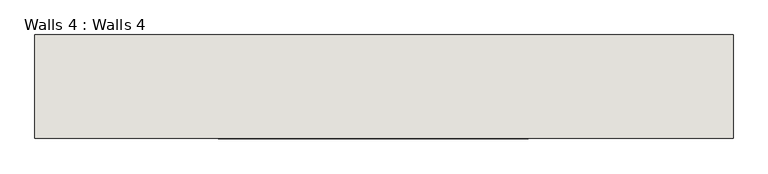
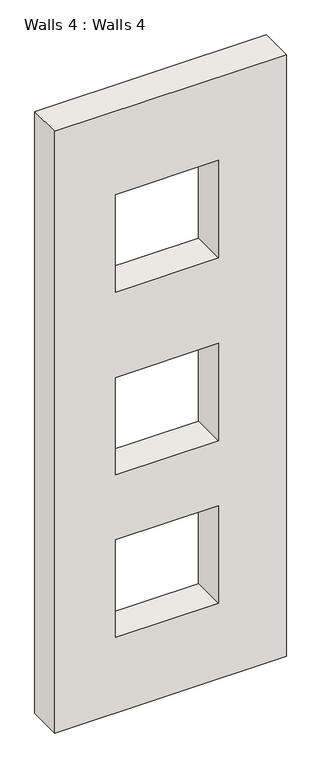
"""IFC4 building model written with IfcOpenShell, lengths in millimetres: wall geometry, Walls 4 : Walls 4."""

from ifc_helpers import new_model, si_unit, frame, origin, place, context, project, spatial, polyline, outline, extrude, source, transform, mapped, element, save


def walls_4_walls_4_1aaea7ad(model_context):
    return source(origin(), model_context, "Body", "SweptSolid", [
        extrude(outline(polyline([(5648.0, -13721.6569137), (5648.0, -15779.6883357), (0.0, -15779.6883357), (0.0, -13721.6569137), (5648.0, -13721.6569137)]), holes=[polyline([(4865.4243496, -14325.0360756), (3951.0243496, -14325.0360756), (3951.0243496, -15239.4360756), (4865.4243496, -15239.4360756), (4865.4243496, -14325.0360756)]), polyline([(3147.9411098, -14325.0360756), (2233.5411098, -14325.0360756), (2233.5411098, -15239.4360756), (3147.9411098, -15239.4360756), (3147.9411098, -14325.0360756)]), polyline([(1623.9411098, -14325.0360756), (709.5411098, -14325.0360756), (709.5411098, -15239.4360756), (1623.9411098, -15239.4360756), (1623.9411098, -14325.0360756)])]), frame((0.0, -20740.5210337, 0.0), z_axis=(0.0, 1.0, 0.0), x_axis=(0.0, 0.0, 1.0)), (0.0, 0.0, 1.0), 304.8),
    ])


if __name__ == "__main__":
    model = new_model("IFC4")
    model_context = context("Model", 3, world=origin())
    ifc_project = project(units=[si_unit("LENGTHUNIT", "METRE", prefix="MILLI")], contexts=[model_context])
    site = spatial("IfcSite", under=ifc_project)
    building = spatial("IfcBuilding", under=site)
    placement = place(None, origin())
    walls_4_walls_4_shape = walls_4_walls_4_1aaea7ad(model_context)
    element("IfcWall", 1, ObjectType="Walls 4 : Walls 4", at=placement, inside=building, context=model_context, shape_type="MappedRepresentation", body=[
        mapped(walls_4_walls_4_shape, transform((0.0, 0.0, 0.0), x_axis=(1.0, 0.0, 0.0), y_axis=(0.0, 1.0, 0.0), z_axis=(0.0, 0.0, 1.0))),
    ])
    save(model, "model.ifc")

# Revit data of these elements
# Element 1 (IfcWall, "Walls 4 : Walls 4")
#   Materials on its faces: "Default Wall"
# Materials
#   "Default Wall": colour RGB 80 80 80, transparency 0
